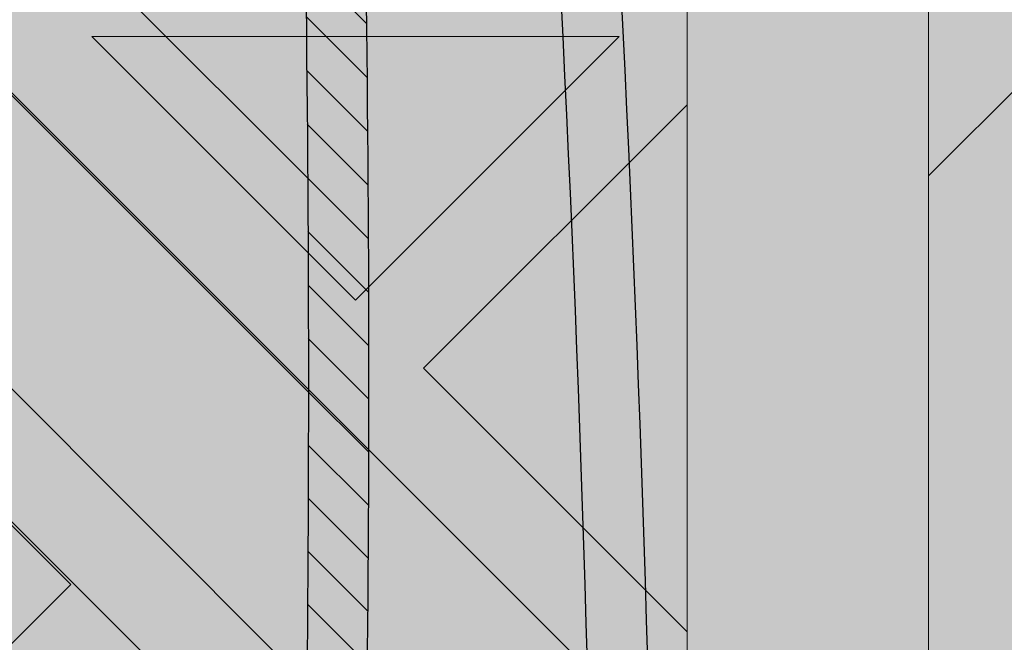
# Model space of a CAD drawing. Units: inches. Extents: x 844 to 2234, y 346 to 1084.
# Tile 36 of 93: x 1260.074 to 1262.676, y 697.583 to 699.229. Entities that reach past the tile are written whole.
import ezdxf

# ---------------------------------------------------------------- set-up
doc = ezdxf.new("R2010")
doc.units = ezdxf.units.IN
doc.header["$MEASUREMENT"] = 0
doc.layers.add('furniture', color=8, linetype='Continuous', lineweight=18)
doc.layers.add('RA-AP-01$0$INT', color=35, linetype='Continuous', lineweight=5)
doc.layers.add('RA-AP-01$0$FURN', color=3, linetype='Continuous')
doc.layers.add('RA-AP-01$0$WOOD', color=64, linetype='Continuous')

# ---------------------------------------------------------------- blocks, each defined once
blk = doc.blocks.new('A$C18D01794')
at = {"layer": 'RA-AP-01$0$INT'}
h = blk.add_hatch(color=256, dxfattribs=at)
h.paths.add_polyline_path([(4.50521, -7.5855), (4.46935, -7.54964), (4.50521, -7.51378), (4.50521, -7.38196), (4.46935, -7.34611), (4.50521, -7.31025), (4.50521, -7.17843), (4.46935, -7.14257), (4.50521, -7.10671), (4.47692, -7.10671), (4.45521, -7.12843), (4.43349, -7.10671), (4.40521, -7.10671), (4.44106, -7.14257), (4.40521, -7.17843), (4.40521, -7.31025), (4.44106, -7.34611), (4.40521, -7.38196), (4.40521, -7.51378), (4.44106, -7.54964), (4.40521, -7.5855), (4.40521, -7.71732), (4.44106, -7.75318), (4.40521, -7.78903), (4.40521, -8.00671), (4.64435, -8.00671), (4.68021, -7.97085), (4.71606, -8.00671), (4.86935, -8.00671), (4.90521, -7.97085), (4.94106, -8.00671), (5.09435, -8.00671), (5.13021, -7.97085), (5.16606, -8.00671), (5.40521, -8.00671), (5.40521, -7.78903), (5.36935, -7.75318), (5.40521, -7.71732), (5.40521, -7.5855), (5.36935, -7.54964), (5.40521, -7.51378), (5.40521, -7.38196), (5.36935, -7.34611), (5.40521, -7.31025), (5.40521, -7.17843), (5.36935, -7.14257), (5.40521, -7.10671), (5.37692, -7.10671), (5.35521, -7.12843), (5.33349, -7.10671), (5.30521, -7.10671), (5.34106, -7.14257), (5.30521, -7.17843), (5.30521, -7.31025), (5.34106, -7.34611), (5.30521, -7.38196), (5.30521, -7.51378), (5.34106, -7.54964), (5.30521, -7.5855), (5.30521, -7.71732), (5.34106, -7.75318), (5.30521, -7.78903), (5.30521, -7.90671), (5.16606, -7.90671), (5.13021, -7.94257), (5.09435, -7.90671), (4.94106, -7.90671), (4.90521, -7.94257), (4.86935, -7.90671), (4.71606, -7.90671), (4.68021, -7.94257), (4.64435, -7.90671), (4.50521, -7.90671), (4.50521, -7.78903), (4.46935, -7.75318), (4.50521, -7.71732)])
h.paths.add_polyline_path([(4.48521, -7.70903), (4.45521, -7.73903), (4.42521, -7.70903), (4.42521, -7.59378), (4.45521, -7.56378), (4.48521, -7.59378)], flags=16)
h.paths.add_polyline_path([(4.45521, -7.76732), (4.48521, -7.79732), (4.48521, -7.91257), (4.45521, -7.94257), (4.42521, -7.91257), (4.42521, -7.79732)], flags=16)
h.paths.add_polyline_path([(4.45521, -7.5355), (4.42521, -7.5055), (4.42521, -7.39025), (4.45521, -7.36025), (4.48521, -7.39025), (4.48521, -7.5055)], flags=16)
h.paths.add_polyline_path([(4.49935, -7.92671), (4.63606, -7.92671), (4.66606, -7.95671), (4.63606, -7.98671), (4.49935, -7.98671), (4.46935, -7.95671)], flags=16)
h.paths.add_polyline_path([(4.42521, -7.94085), (4.47106, -7.98671), (4.42521, -7.98671)], flags=16)
h.paths.add_polyline_path([(4.45521, -7.33196), (4.42521, -7.30196), (4.42521, -7.18671), (4.45521, -7.15671), (4.48521, -7.18671), (4.48521, -7.30196)], flags=16)
h.paths.add_polyline_path([(4.72435, -7.92671), (4.86106, -7.92671), (4.89106, -7.95671), (4.86106, -7.98671), (4.72435, -7.98671), (4.69435, -7.95671)], flags=16)
h.paths.add_polyline_path([(4.91935, -7.95671), (4.94935, -7.92671), (5.08606, -7.92671), (5.11606, -7.95671), (5.08606, -7.98671), (4.94935, -7.98671)], flags=16)
h.paths.add_polyline_path([(5.14435, -7.95671), (5.17435, -7.92671), (5.31106, -7.92671), (5.34106, -7.95671), (5.31106, -7.98671), (5.17435, -7.98671)], flags=16)
h.paths.add_polyline_path([(5.32521, -7.59378), (5.35521, -7.56378), (5.38521, -7.59378), (5.38521, -7.70903), (5.35521, -7.73903), (5.32521, -7.70903)], flags=16)
h.paths.add_polyline_path([(5.32521, -7.79732), (5.35521, -7.76732), (5.38521, -7.79732), (5.38521, -7.91257), (5.35521, -7.94257), (5.32521, -7.91257)], flags=16)
h.paths.add_polyline_path([(5.32521, -7.5055), (5.32521, -7.39025), (5.35521, -7.36025), (5.38521, -7.39025), (5.38521, -7.5055), (5.35521, -7.5355)], flags=16)
h.paths.add_polyline_path([(5.32521, -7.30196), (5.32521, -7.18671), (5.35521, -7.15671), (5.38521, -7.18671), (5.38521, -7.30196), (5.35521, -7.33196)], flags=16)
h.paths.add_polyline_path([(5.33935, -7.98671), (5.38521, -7.94085), (5.38521, -7.98671)], flags=16)
h = blk.add_hatch(color=256, dxfattribs=at)
h.paths.add_polyline_path([(4.46935, -7.14257), (4.50521, -7.17843), (4.50521, -7.10671)])
h.paths.add_polyline_path([(4.45521, -7.12843), (4.47692, -7.10671), (4.43349, -7.10671)])
h.paths.add_polyline_path([(4.40521, -7.17843), (4.44106, -7.14257), (4.40521, -7.10671)])
h.paths.add_polyline_path([(4.42521, -7.30196), (4.45521, -7.33196), (4.48521, -7.30196), (4.48521, -7.18671), (4.45521, -7.15671), (4.42521, -7.18671)])
h.paths.add_polyline_path([(4.50521, -7.38196), (4.50521, -7.31025), (4.46935, -7.34611)])
h.paths.add_polyline_path([(4.42521, -7.5055), (4.45521, -7.5355), (4.48521, -7.5055), (4.48521, -7.39025), (4.45521, -7.36025), (4.42521, -7.39025)])
h.paths.add_polyline_path([(4.42521, -7.70903), (4.45521, -7.73903), (4.48521, -7.70903), (4.48521, -7.59378), (4.45521, -7.56378), (4.42521, -7.59378)])
h.paths.add_polyline_path([(4.46935, -7.54964), (4.50521, -7.5855), (4.50521, -7.51378)])
h.paths.add_polyline_path([(4.40521, -7.5855), (4.44106, -7.54964), (4.40521, -7.51378)])
h.paths.add_polyline_path([(4.40521, -7.78903), (4.44106, -7.75318), (4.40521, -7.71732)])
h.paths.add_polyline_path([(4.46935, -7.75318), (4.50521, -7.78903), (4.50521, -7.71732)])
h.paths.add_polyline_path([(4.42521, -7.91257), (4.45521, -7.94257), (4.48521, -7.91257), (4.48521, -7.79732), (4.45521, -7.76732), (4.42521, -7.79732)])
h.paths.add_polyline_path([(4.42521, -7.98671), (4.47106, -7.98671), (4.42521, -7.94085)])
h.paths.add_polyline_path([(4.49935, -7.98671), (4.63606, -7.98671), (4.66606, -7.95671), (4.63606, -7.92671), (4.49935, -7.92671), (4.46935, -7.95671)])
h.paths.add_polyline_path([(4.68021, -7.94257), (4.71606, -7.90671), (4.64435, -7.90671)])
h.paths.add_polyline_path([(4.64435, -8.00671), (4.71606, -8.00671), (4.68021, -7.97085)])
h.paths.add_polyline_path([(4.72435, -7.98671), (4.86106, -7.98671), (4.89106, -7.95671), (4.86106, -7.92671), (4.72435, -7.92671), (4.69435, -7.95671)])
h.paths.add_polyline_path([(4.90521, -7.94257), (4.94106, -7.90671), (4.86935, -7.90671)])
h.paths.add_polyline_path([(4.86935, -8.00671), (4.94106, -8.00671), (4.90521, -7.97085)])
h.paths.add_polyline_path([(4.94935, -7.98671), (5.08606, -7.98671), (5.11606, -7.95671), (5.08606, -7.92671), (4.94935, -7.92671), (4.91935, -7.95671)])
h.paths.add_polyline_path([(5.13021, -7.94257), (5.16606, -7.90671), (5.09435, -7.90671)])
h.paths.add_polyline_path([(5.09435, -8.00671), (5.16606, -8.00671), (5.13021, -7.97085)])
h.paths.add_polyline_path([(5.17435, -7.98671), (5.31106, -7.98671), (5.34106, -7.95671), (5.31106, -7.92671), (5.17435, -7.92671), (5.14435, -7.95671)])
h.paths.add_polyline_path([(5.32521, -7.91257), (5.35521, -7.94257), (5.38521, -7.91257), (5.38521, -7.79732), (5.35521, -7.76732), (5.32521, -7.79732)])
h.paths.add_polyline_path([(5.33935, -7.98671), (5.38521, -7.98671), (5.38521, -7.94085)])
h.paths.add_polyline_path([(5.32521, -7.70903), (5.35521, -7.73903), (5.38521, -7.70903), (5.38521, -7.59378), (5.35521, -7.56378), (5.32521, -7.59378)])
h.paths.add_polyline_path([(5.30521, -7.78903), (5.34106, -7.75318), (5.30521, -7.71732)])
h.paths.add_polyline_path([(5.36935, -7.75318), (5.40521, -7.78903), (5.40521, -7.71732)])
h.paths.add_polyline_path([(5.40521, -7.5855), (5.40521, -7.51378), (5.36935, -7.54964)])
h.paths.add_polyline_path([(5.30521, -7.5855), (5.34106, -7.54964), (5.30521, -7.51378)])
h.paths.add_polyline_path([(5.32521, -7.5055), (5.35521, -7.5355), (5.38521, -7.5055), (5.38521, -7.39025), (5.35521, -7.36025), (5.32521, -7.39025)])
h.paths.add_polyline_path([(5.30521, -7.38196), (5.34106, -7.34611), (5.30521, -7.31025)])
h.paths.add_polyline_path([(5.32521, -7.30196), (5.35521, -7.33196), (5.38521, -7.30196), (5.38521, -7.18671), (5.35521, -7.15671), (5.32521, -7.18671)])
h.paths.add_polyline_path([(5.40458, -7.38134, -0.001218), (5.40521, -7.38111), (5.40521, -7.31025), (5.36935, -7.34611)])
h.paths.add_polyline_path([(5.36935, -7.14257), (5.40521, -7.17843), (5.40521, -7.10671)])
h.paths.add_polyline_path([(5.35521, -7.12843), (5.37692, -7.10671), (5.33349, -7.10671)])
h.paths.add_polyline_path([(5.30521, -7.17843), (5.34106, -7.14257), (5.30521, -7.10671)])
blk.add_hatch(color=256, dxfattribs=at).paths.add_polyline_path([(4.50521, -7.90671), (5.30521, -7.90671), (5.30521, -7.10671), (5.25521, -7.10671), (5.25521, -7.85671), (4.55521, -7.85671), (4.55521, -7.10671), (4.50521, -7.10671)])
h = blk.add_hatch(color=256, dxfattribs=at)
h.paths.add_polyline_path([(4.58592, -7.85671), (4.6142, -7.85671), (4.66885, -7.80207), (4.72349, -7.85671), (4.77177, -7.85671), (4.82642, -7.80207), (4.86278, -7.83843), (4.8445, -7.85671), (4.86278, -7.85671), (4.90521, -7.81429), (4.94763, -7.85671), (4.96592, -7.85671), (4.94763, -7.83843), (4.98399, -7.80207), (5.03864, -7.85671), (5.08692, -7.85671), (5.14157, -7.80207), (5.19621, -7.85671), (5.2245, -7.85671), (4.90521, -7.53742)])
h.paths.add_polyline_path([(4.89521, -7.57571), (4.89521, -7.685), (4.84056, -7.63035)], flags=16)
h.paths.add_polyline_path([(4.91521, -7.57571), (4.96985, -7.63035), (4.91521, -7.685)], flags=16)
h.paths.add_polyline_path([(4.82642, -7.64449), (4.88106, -7.69914), (4.77177, -7.69914)], flags=16)
h.paths.add_polyline_path([(4.98399, -7.64449), (5.03864, -7.69914), (4.92935, -7.69914)], flags=16)
h.paths.add_polyline_path([(4.88106, -7.71914), (4.82642, -7.77378), (4.77177, -7.71914)], flags=16)
h.paths.add_polyline_path([(4.92935, -7.71914), (5.03864, -7.71914), (4.98399, -7.77378)], flags=16)
h.paths.add_polyline_path([(4.89521, -7.73328), (4.89521, -7.806), (4.87692, -7.82429), (4.84056, -7.78793)], flags=16)
h.paths.add_polyline_path([(4.91521, -7.73328), (4.96985, -7.78793), (4.93349, -7.82429), (4.91521, -7.806)], flags=16)
h.paths.add_polyline_path([(4.75763, -7.73328), (4.81228, -7.78793), (4.75763, -7.84257)], flags=16)
h.paths.add_polyline_path([(4.73763, -7.73328), (4.73763, -7.84257), (4.68299, -7.78793)], flags=16)
h.paths.add_polyline_path([(5.05278, -7.73328), (5.05278, -7.84257), (4.99814, -7.78793)], flags=16)
h.paths.add_polyline_path([(5.07278, -7.73328), (5.12742, -7.78793), (5.07278, -7.84257)], flags=16)
h.paths.add_polyline_path([(4.93592, -7.50671), (5.25521, -7.826), (5.25521, -7.79772), (5.20056, -7.74307), (5.25521, -7.68843), (5.25521, -7.64014), (5.20056, -7.5855), (5.23692, -7.54914), (5.25521, -7.56742), (5.25521, -7.54914), (5.21278, -7.50671), (5.25521, -7.46429), (5.25521, -7.446), (5.23692, -7.46429), (5.20056, -7.42793), (5.25521, -7.37328), (5.25521, -7.325), (5.20056, -7.27035), (5.25521, -7.21571), (5.25521, -7.18742)])
h.paths.add_polyline_path([(5.04299, -7.42793), (5.09763, -7.37328), (5.09763, -7.48257)], flags=16)
h.paths.add_polyline_path([(5.02885, -7.44207), (5.08349, -7.49671), (4.9742, -7.49671)], flags=16)
h.paths.add_polyline_path([(5.11763, -7.37328), (5.17228, -7.42793), (5.11763, -7.48257)], flags=16)
h.paths.add_polyline_path([(5.08349, -7.51671), (5.02885, -7.57136), (4.9742, -7.51671)], flags=16)
h.paths.add_polyline_path([(5.13177, -7.35914), (5.18642, -7.41378), (5.24106, -7.35914)], flags=17)
h.paths.add_polyline_path([(5.13177, -7.49671), (5.18642, -7.44207), (5.22278, -7.47843), (5.2045, -7.49671)], flags=16)
h.paths.add_polyline_path([(5.09763, -7.53085), (5.09763, -7.64014), (5.04299, -7.5855)], flags=16)
h.paths.add_polyline_path([(5.13177, -7.33914), (5.24106, -7.33914), (5.18642, -7.28449)], flags=17)
h.paths.add_polyline_path([(5.13177, -7.51671), (5.2045, -7.51671), (5.22278, -7.535), (5.18642, -7.57136)], flags=16)
h.paths.add_polyline_path([(5.11763, -7.53085), (5.17228, -7.5855), (5.11763, -7.64014)], flags=16)
h.paths.add_polyline_path([(5.18642, -7.59964), (5.24106, -7.65429), (5.13177, -7.65429)], flags=16)
h.paths.add_polyline_path([(5.13177, -7.67429), (5.24106, -7.67429), (5.18642, -7.72893)], flags=16)
h.paths.add_polyline_path([(5.25521, -7.126), (5.25521, -7.10671), (4.55521, -7.10671), (4.55521, -7.126), (4.90521, -7.476)])
h.paths.add_polyline_path([(4.98399, -7.36893), (4.92935, -7.31429), (5.03864, -7.31429)], flags=16)
h.paths.add_polyline_path([(4.96985, -7.38307), (4.91521, -7.43772), (4.91521, -7.32843)], flags=16)
h.paths.add_polyline_path([(4.92935, -7.29429), (4.98399, -7.23964), (5.03864, -7.29429)], flags=16)
h.paths.add_polyline_path([(5.05278, -7.28014), (4.99814, -7.2255), (5.05278, -7.17085)], flags=16)
h.paths.add_polyline_path([(5.07278, -7.28014), (5.07278, -7.17085), (5.12742, -7.2255)], flags=16)
h.paths.add_polyline_path([(4.89521, -7.43772), (4.84056, -7.38307), (4.89521, -7.32843)], flags=16)
h.paths.add_polyline_path([(4.91521, -7.28014), (4.91521, -7.20742), (4.93349, -7.18914), (4.96985, -7.2255)], flags=16)
h.paths.add_polyline_path([(4.88106, -7.31429), (4.82642, -7.36893), (4.77177, -7.31429)], flags=16)
h.paths.add_polyline_path([(4.89521, -7.28014), (4.84056, -7.2255), (4.87692, -7.18914), (4.89521, -7.20742)], flags=16)
h.paths.add_polyline_path([(4.98399, -7.21136), (4.94763, -7.175), (4.96592, -7.15671), (5.03864, -7.15671)], flags=16)
h.paths.add_polyline_path([(4.88106, -7.29429), (4.77177, -7.29429), (4.82642, -7.23964)], flags=16)
h.paths.add_polyline_path([(4.90521, -7.19914), (4.86278, -7.15671), (4.94763, -7.15671)], flags=16)
h.paths.add_polyline_path([(5.14157, -7.21136), (5.08692, -7.15671), (5.19621, -7.15671)], flags=16)
h.paths.add_polyline_path([(4.82642, -7.21136), (4.77177, -7.15671), (4.8445, -7.15671), (4.86278, -7.175)], flags=16)
h.paths.add_polyline_path([(4.81228, -7.2255), (4.75763, -7.28014), (4.75763, -7.17085)], flags=16)
h.paths.add_polyline_path([(4.73763, -7.28014), (4.68299, -7.2255), (4.73763, -7.17085)], flags=16)
h.paths.add_polyline_path([(4.72349, -7.15671), (4.66885, -7.21136), (4.6142, -7.15671)], flags=16)
h.paths.add_polyline_path([(4.59763, -7.50671), (4.55521, -7.54914), (4.55521, -7.56742), (4.57349, -7.54914), (4.60985, -7.5855), (4.55521, -7.64014), (4.55521, -7.68843), (4.60985, -7.74307), (4.55521, -7.79772), (4.55521, -7.826), (4.8745, -7.50671), (4.55521, -7.18742), (4.55521, -7.21571), (4.60985, -7.27035), (4.55521, -7.325), (4.55521, -7.37328), (4.60985, -7.42793), (4.57349, -7.46429), (4.55521, -7.446), (4.55521, -7.46429)])
h.paths.add_polyline_path([(4.71278, -7.48257), (4.71278, -7.37328), (4.76742, -7.42793)], flags=16)
h.paths.add_polyline_path([(4.72692, -7.49671), (4.78157, -7.44207), (4.83621, -7.49671)], flags=16)
h.paths.add_polyline_path([(4.69278, -7.48257), (4.63814, -7.42793), (4.69278, -7.37328)], flags=16)
h.paths.add_polyline_path([(4.72692, -7.51671), (4.83621, -7.51671), (4.78157, -7.57136)], flags=16)
h.paths.add_polyline_path([(4.67864, -7.49671), (4.60592, -7.49671), (4.58763, -7.47843), (4.62399, -7.44207)], flags=16)
h.paths.add_polyline_path([(4.71278, -7.53085), (4.76742, -7.5855), (4.71278, -7.64014)], flags=16)
h.paths.add_polyline_path([(4.67864, -7.51671), (4.62399, -7.57136), (4.58763, -7.535), (4.60592, -7.51671)], flags=16)
h.paths.add_polyline_path([(4.69278, -7.53085), (4.69278, -7.64014), (4.63814, -7.5855)], flags=16)
h.paths.add_polyline_path([(4.62399, -7.41378), (4.67864, -7.35914), (4.56935, -7.35914)], flags=17)
h.paths.add_polyline_path([(4.62399, -7.59964), (4.67864, -7.65429), (4.56935, -7.65429)], flags=16)
h.paths.add_polyline_path([(4.67864, -7.33914), (4.62399, -7.28449), (4.56935, -7.33914)], flags=17)
h.paths.add_polyline_path([(4.67864, -7.67429), (4.62399, -7.72893), (4.56935, -7.67429)], flags=16)
h = blk.add_hatch(color=256, dxfattribs=at)
h.paths.add_polyline_path([(4.90521, -7.53742), (4.8745, -7.50671), (4.55521, -7.826), (4.55521, -7.85671), (4.58592, -7.85671)])
h.paths.add_polyline_path([(4.93592, -7.50671), (4.90521, -7.53742), (5.2245, -7.85671), (5.25521, -7.85671), (5.25521, -7.826)])
h.paths.add_polyline_path([(5.25521, -7.18742), (5.25521, -7.126), (4.90521, -7.476), (4.93592, -7.50671)])
h.paths.add_polyline_path([(4.8745, -7.50671), (4.90521, -7.476), (4.55521, -7.126), (4.55521, -7.18742)])
h = blk.add_hatch(color=256, dxfattribs=at)
h.paths.add_polyline_path([(4.89521, -7.32843), (4.84056, -7.38307), (4.89521, -7.43772)])
h.paths.add_polyline_path([(4.91521, -7.43772), (4.96985, -7.38307), (4.91521, -7.32843)])
h.paths.add_polyline_path([(4.92935, -7.31429), (4.98399, -7.36893), (5.03864, -7.31429)])
h.paths.add_polyline_path([(5.03864, -7.29429), (4.98399, -7.23964), (4.92935, -7.29429)])
h.paths.add_polyline_path([(4.96985, -7.2255), (4.93349, -7.18914), (4.91521, -7.20742), (4.91521, -7.28014)])
h.paths.add_polyline_path([(4.96592, -7.15671), (4.94763, -7.175), (4.98399, -7.21136), (5.03864, -7.15671)])
h.paths.add_polyline_path([(4.99814, -7.2255), (5.05278, -7.28014), (5.05278, -7.17085)])
h.paths.add_polyline_path([(5.07278, -7.28014), (5.12742, -7.2255), (5.07278, -7.17085)])
h.paths.add_polyline_path([(5.19621, -7.15671), (5.08692, -7.15671), (5.14157, -7.21136)])
h.paths.add_polyline_path([(4.86278, -7.15671), (4.90521, -7.19914), (4.94763, -7.15671)])
h.paths.add_polyline_path([(4.89521, -7.28014), (4.89521, -7.20742), (4.87692, -7.18914), (4.84056, -7.2255)])
h.paths.add_polyline_path([(4.82642, -7.23964), (4.77177, -7.29429), (4.88106, -7.29429)])
h.paths.add_polyline_path([(4.77177, -7.31429), (4.82642, -7.36893), (4.88106, -7.31429)])
h.paths.add_polyline_path([(4.75763, -7.28014), (4.81228, -7.2255), (4.75763, -7.17085)])
h.paths.add_polyline_path([(4.86278, -7.175), (4.8445, -7.15671), (4.77177, -7.15671), (4.82642, -7.21136)])
h.paths.add_polyline_path([(4.68299, -7.2255), (4.73763, -7.28014), (4.73763, -7.17085)])
h.paths.add_polyline_path([(4.72349, -7.15671), (4.6142, -7.15671), (4.66885, -7.21136)])
h = blk.add_hatch(color=256, dxfattribs=at)
h.paths.add_polyline_path([(4.78157, -7.44207), (4.83621, -7.49671), (4.72692, -7.49671)])
h.paths.add_polyline_path([(4.83621, -7.51671), (4.78157, -7.57136), (4.72692, -7.51671)])
h.paths.add_polyline_path([(4.76742, -7.5855), (4.71278, -7.64014), (4.71278, -7.53085)])
h.paths.add_polyline_path([(4.69278, -7.53085), (4.69278, -7.64014), (4.63814, -7.5855)])
h.paths.add_polyline_path([(4.67864, -7.51671), (4.62399, -7.57136), (4.58763, -7.535), (4.60592, -7.51671)])
h.paths.add_polyline_path([(4.57349, -7.54914), (4.60985, -7.5855), (4.55521, -7.64014), (4.55521, -7.56742)])
h.paths.add_polyline_path([(4.62399, -7.59964), (4.67864, -7.65429), (4.56935, -7.65429)])
h.paths.add_polyline_path([(4.67864, -7.67429), (4.62399, -7.72893), (4.56935, -7.67429)])
h.paths.add_polyline_path([(4.60985, -7.74307), (4.55521, -7.79772), (4.55521, -7.68843)])
h.paths.add_polyline_path([(4.59763, -7.50671), (4.55521, -7.54914), (4.55521, -7.46429)])
h.paths.add_polyline_path([(4.67864, -7.49671), (4.60592, -7.49671), (4.58763, -7.47843), (4.62399, -7.44207)])
h.paths.add_polyline_path([(4.69278, -7.37328), (4.69278, -7.48257), (4.63814, -7.42793)])
h.paths.add_polyline_path([(4.76742, -7.42793), (4.71278, -7.48257), (4.71278, -7.37328)])
h.paths.add_polyline_path([(4.67864, -7.35914), (4.62399, -7.41378), (4.56935, -7.35914)])
h.paths.add_polyline_path([(4.60985, -7.42793), (4.57349, -7.46429), (4.55521, -7.446), (4.55521, -7.37328)])
h.paths.add_polyline_path([(4.62399, -7.28449), (4.67864, -7.33914), (4.56935, -7.33914)])
h.paths.add_polyline_path([(4.60985, -7.27035), (4.55521, -7.325), (4.55521, -7.21571)])
for p, q in [((4.55521, -7.10671), (4.55521, -7.85671)), ((4.90521, -7.476), (4.55521, -7.126)), ((4.73763, -7.17085), (4.68299, -7.2255)), ((4.8745, -7.50671), (4.55521, -7.18742)), ((4.55521, -7.21571), (4.60985, -7.27035)), ((4.55521, -7.325), (4.55521, -7.21571)), ((4.68299, -7.2255), (4.73763, -7.28014)), ((4.55521, -7.325), (4.60985, -7.27035)), ((4.56935, -7.33914), (4.62399, -7.28449)), ((4.62399, -7.28449), (4.67864, -7.33914)), ((4.50521, -7.31025), (4.46935, -7.34611)), ((4.67864, -7.33914), (4.56935, -7.33914))]:
    blk.add_line(p, q, dxfattribs=at)
blk.add_lwpolyline([(5.30521, -7.10671), (5.30521, -7.90671), (4.50521, -7.90671), (4.50521, -7.10671)], dxfattribs=at)
blk = doc.blocks.new('A$C32926AE1')
at = {"layer": 'RA-AP-01$0$WOOD'}
h = blk.add_hatch(color=256, dxfattribs=at)
h.dxf.hatch_style = 1
h.paths.add_polyline_path([(5.15743, 4.57348, -0.100949), (5.1554, 4.59337, -0.184266), (5.17225, 4.6388, 0.205661), (5.17956, 4.66132, 0.361434), (5.13435, 4.70652, 0.205661), (5.11183, 4.69921, -0.184266), (5.0664, 4.68237, -0.105531), (5.04566, 4.68467, 0.156764), (4.76389, 4.68467, -0.105531), (4.74314, 4.68237, -0.184266), (4.69771, 4.69921, 0.205661), (4.67519, 4.70652, 0.361434), (4.62998, 4.66132, 0.205661), (4.63729, 4.6388, -0.184266), (4.65414, 4.59337, -0.100949), (4.65211, 4.57348, 0.02141), (4.62975, 4.15671, 0.02141), (4.65211, 3.73994, -0.100949), (4.65414, 3.72006, -0.184266), (4.63729, 3.67463, 0.205661), (4.62998, 3.65211, 0.361434), (4.67519, 3.6069, 0.205661), (4.69771, 3.61421, -0.184266), (4.74314, 3.63106, -0.105531), (4.76389, 3.62875, 0.156764), (5.04566, 3.62875, -0.105531), (5.0664, 3.63106, -0.184266), (5.11183, 3.61421, 0.205661), (5.13435, 3.6069, 0.361434), (5.17956, 3.65211, 0.205661), (5.17225, 3.67463, -0.184266), (5.1554, 3.72006, -0.100949), (5.15743, 3.73994, 0.02141), (5.17979, 4.15671, 0.02141)])
h.paths.add_polyline_path([(4.63975, 4.15671, 0.021354), (4.66197, 3.74189, -0.094076), (4.66414, 3.71961, -0.182482), (4.64481, 3.66804, 0.205661), (4.63994, 3.65302, 0.361434), (4.67611, 3.61686, 0.205661), (4.69112, 3.62173, -0.182482), (4.7427, 3.64106, -0.102989), (4.76699, 3.63826, 0.156709), (5.04255, 3.63826, -0.102989), (5.06685, 3.64106, -0.182482), (5.11842, 3.62173, 0.205661), (5.13344, 3.61686, 0.361434), (5.1696, 3.65302, 0.205661), (5.16473, 3.66804, -0.182482), (5.1454, 3.71961, -0.094076), (5.14757, 3.74189, 0.021354), (5.16979, 4.15671, 0.021354), (5.14757, 4.57154, -0.094076), (5.1454, 4.59381, -0.182482), (5.16473, 4.64539, 0.205661), (5.1696, 4.6604, 0.361434), (5.13344, 4.69657, 0.205661), (5.11842, 4.69169, -0.182482), (5.06685, 4.67236, -0.102989), (5.04255, 4.67517, 0.156709), (4.76699, 4.67517, -0.102989), (4.7427, 4.67236, -0.182482), (4.69112, 4.69169, 0.205661), (4.67611, 4.69657, 0.361434), (4.63994, 4.6604, 0.205661), (4.64481, 4.64539, -0.182482), (4.66414, 4.59381, -0.094076), (4.66197, 4.57154, 0.021354)], flags=16)
h.paths.add_polyline_path([(5.12979, 4.43217, -0.014166), (5.13015, 4.15693, -0.014166), (5.12979, 3.88169, -0.078525), (5.1098, 3.75514, 0.094597), (5.10541, 3.7179, 0.104317), (5.11607, 3.67039, 0.104317), (5.06856, 3.68105, 0.094597), (5.03132, 3.67666, -0.158024), (4.77823, 3.67666, 0.094597), (4.74098, 3.68105, 0.104317), (4.69347, 3.67039, 0.104317), (4.70413, 3.7179, 0.094597), (4.69975, 3.75514, -0.078525), (4.67975, 3.88169, -0.014166), (4.67939, 4.15693, -0.014166), (4.67975, 4.43217, -0.078525), (4.69975, 4.55871, 0.094597), (4.70413, 4.59596, 0.104317), (4.69347, 4.64347, 0.104317), (4.74098, 4.6328, 0.094597), (4.77823, 4.63719, -0.158024), (5.03132, 4.63719, 0.094597), (5.06856, 4.6328, 0.104317), (5.11607, 4.64347, 0.104317), (5.10541, 4.59596, 0.094597), (5.1098, 4.55871, -0.078525)], flags=0)
h.paths.add_polyline_path([(5.11979, 4.43226, -0.0142), (5.12016, 4.15693, -0.0142), (5.11979, 3.8816, -0.078489), (5.10027, 3.75819, 0.094014), (5.09541, 3.71748, 0.060627), (5.09962, 3.68684, 0.060627), (5.06898, 3.69105, 0.094014), (5.02827, 3.68619, -0.158071), (4.78127, 3.68619, 0.094014), (4.74056, 3.69105, 0.060627), (4.70993, 3.68684, 0.060627), (4.71413, 3.71748, 0.094014), (4.70927, 3.75819, -0.078489), (4.68975, 3.8816, -0.0142), (4.68939, 4.15693, -0.0142), (4.68975, 4.43226, -0.078489), (4.70927, 4.55566, 0.094014), (4.71413, 4.59638, 0.060627), (4.70993, 4.62701, 0.060627), (4.74056, 4.62281, 0.094014), (4.78127, 4.62767, -0.158071), (5.02827, 4.62767, 0.094014), (5.06898, 4.62281, 0.060627), (5.09962, 4.62701, 0.060627), (5.09541, 4.59638, 0.094014), (5.10027, 4.55566, -0.078489)], flags=0)
h.paths.add_polyline_path([(5.06979, 4.43022, -0.014242), (5.07017, 4.15693, -0.014242), (5.06979, 3.88364, -0.080061), (5.05266, 3.77346, 0.052642), (5.04591, 3.74055, 0.052642), (5.013, 3.7338, -0.158303), (4.79655, 3.7338, 0.052642), (4.76363, 3.74055, 0.052642), (4.75688, 3.77346, -0.080061), (4.73975, 3.88364, -0.014242), (4.73937, 4.15693, -0.014242), (4.73975, 4.43022, -0.080061), (4.75688, 4.54039, 0.052642), (4.76363, 4.5733, 0.052642), (4.79655, 4.58006, -0.158303), (5.013, 4.58006, 0.052642), (5.04591, 4.5733, 0.052642), (5.05266, 4.54039, -0.080061)], flags=0)
h.paths.add_polyline_path([(5.04979, 4.43038, -0.01431), (5.05018, 4.15693, -0.01431), (5.04979, 3.88347, -0.080069), (5.03362, 3.77958, 0.030626), (5.02824, 3.75822, 0.030626), (5.00688, 3.75284, -0.158398), (4.80266, 3.75284, 0.030626), (4.7813, 3.75822, 0.030626), (4.77592, 3.77958, -0.080069), (4.75975, 3.88347, -0.01431), (4.75936, 4.15693, -0.01431), (4.75975, 4.43038, -0.080069), (4.77592, 4.53427, 0.030626), (4.7813, 4.55564, 0.030626), (4.80266, 4.56102, -0.158398), (5.00688, 4.56102, 0.030626), (5.02824, 4.55564, 0.030626), (5.03362, 4.53427, -0.080069)], flags=0)
h.paths.add_polyline_path([(4.99977, 4.42817, -0.014344), (5.0002, 4.15693, -0.014344), (4.99977, 3.88568, -0.078464), (4.98736, 3.7991, -0.150605), (4.82219, 3.7991, -0.078464), (4.80978, 3.88568, -0.014344), (4.80934, 4.15693, -0.014344), (4.80978, 4.42817, -0.078464), (4.82219, 4.51475, -0.150605), (4.98736, 4.51475, -0.078464)], flags=0)
h.paths.add_polyline_path([(4.97976, 4.42764, -0.014377), (4.98021, 4.15693, -0.014377), (4.97976, 3.88621, -0.068924), (4.97118, 3.81528, -0.129665), (4.83836, 3.81528, -0.068924), (4.82979, 3.88621, -0.014377), (4.82934, 4.15693, -0.014377), (4.82979, 4.42764, -0.068924), (4.83836, 4.49858, -0.129665), (4.97118, 4.49858, -0.068924)], flags=0)
h = blk.add_hatch(color=256, dxfattribs=at)
h.dxf.hatch_style = 1
h.paths.add_polyline_path([(5.1454, 4.59381, -0.182482), (5.16473, 4.64539, 0.205661), (5.1696, 4.6604, 0.361434), (5.13344, 4.69657, 0.205661), (5.11842, 4.69169, -0.182482), (5.06685, 4.67236, -0.102989), (5.04255, 4.67517, 0.156709), (4.76699, 4.67517, -0.102989), (4.7427, 4.67236, -0.182482), (4.69112, 4.69169, 0.205661), (4.67611, 4.69657, 0.361434), (4.63994, 4.6604, 0.205661), (4.64481, 4.64539, -0.182482), (4.66414, 4.59381, -0.094076), (4.66197, 4.57154, 0.021354), (4.63975, 4.15671, 0.021354), (4.66197, 3.74189, -0.094076), (4.66414, 3.71961, -0.182482), (4.64481, 3.66804, 0.205661), (4.63994, 3.65302, 0.361434), (4.67611, 3.61686, 0.205661), (4.69112, 3.62173, -0.182482), (4.7427, 3.64106, -0.102989), (4.76699, 3.63826, 0.156709), (5.04255, 3.63826, -0.102989), (5.06685, 3.64106, -0.182482), (5.11842, 3.62173, 0.205661), (5.13344, 3.61686, 0.361434), (5.1696, 3.65302, 0.205661), (5.16473, 3.66804, -0.182482), (5.1454, 3.71961, -0.094076), (5.14757, 3.74189, 0.021354), (5.16979, 4.15671, 0.021354), (5.14757, 4.57154, -0.094076)])
h.paths.add_polyline_path([(5.1098, 4.55871, -0.078525), (5.12979, 4.43217, -0.014166), (5.13015, 4.15693, -0.014166), (5.12979, 3.88169, -0.078525), (5.1098, 3.75514, 0.094597), (5.10541, 3.7179, 0.104317), (5.11607, 3.67039, 0.104317), (5.06856, 3.68105, 0.094597), (5.03132, 3.67666, -0.158024), (4.77823, 3.67666, 0.094597), (4.74098, 3.68105, 0.104317), (4.69347, 3.67039, 0.104317), (4.70413, 3.7179, 0.094597), (4.69975, 3.75514, -0.078525), (4.67975, 3.88169, -0.014166), (4.67939, 4.15693, -0.014166), (4.67975, 4.43217, -0.078525), (4.69975, 4.55871, 0.094597), (4.70413, 4.59596, 0.104317), (4.69347, 4.64347, 0.104317), (4.74098, 4.6328, 0.094597), (4.77823, 4.63719, -0.158024), (5.03132, 4.63719, 0.094597), (5.06856, 4.6328, 0.104317), (5.11607, 4.64347, 0.104317), (5.10541, 4.59596, 0.094597)], flags=16)
h.paths.add_polyline_path([(5.10027, 4.55566, -0.078489), (5.11979, 4.43226, -0.0142), (5.12016, 4.15693, -0.0142), (5.11979, 3.8816, -0.078489), (5.10027, 3.75819, 0.094014), (5.09541, 3.71748, 0.060627), (5.09962, 3.68684, 0.060627), (5.06898, 3.69105, 0.094014), (5.02827, 3.68619, -0.158071), (4.78127, 3.68619, 0.094014), (4.74056, 3.69105, 0.060627), (4.70993, 3.68684, 0.060627), (4.71413, 3.71748, 0.094014), (4.70927, 3.75819, -0.078489), (4.68975, 3.8816, -0.0142), (4.68939, 4.15693, -0.0142), (4.68975, 4.43226, -0.078489), (4.70927, 4.55566, 0.094014), (4.71413, 4.59638, 0.060627), (4.70993, 4.62701, 0.060627), (4.74056, 4.62281, 0.094014), (4.78127, 4.62767, -0.158071), (5.02827, 4.62767, 0.094014), (5.06898, 4.62281, 0.060627), (5.09962, 4.62701, 0.060627), (5.09541, 4.59638, 0.094014)], flags=0)
h.paths.add_polyline_path([(5.04591, 4.5733, 0.052642), (5.05266, 4.54039, -0.080061), (5.06979, 4.43022, -0.014242), (5.07017, 4.15693, -0.014242), (5.06979, 3.88364, -0.080061), (5.05266, 3.77346, 0.052642), (5.04591, 3.74055, 0.052642), (5.013, 3.7338, -0.158303), (4.79655, 3.7338, 0.052642), (4.76363, 3.74055, 0.052642), (4.75688, 3.77346, -0.080061), (4.73975, 3.88364, -0.014242), (4.73937, 4.15693, -0.014242), (4.73975, 4.43022, -0.080061), (4.75688, 4.54039, 0.052642), (4.76363, 4.5733, 0.052642), (4.79655, 4.58006, -0.158303), (5.013, 4.58006, 0.052642)], flags=0)
h.paths.add_polyline_path([(5.02824, 4.55564, 0.030626), (5.03362, 4.53427, -0.080069), (5.04979, 4.43038, -0.01431), (5.05018, 4.15693, -0.01431), (5.04979, 3.88347, -0.080069), (5.03362, 3.77958, 0.030626), (5.02824, 3.75822, 0.030626), (5.00688, 3.75284, -0.158398), (4.80266, 3.75284, 0.030626), (4.7813, 3.75822, 0.030626), (4.77592, 3.77958, -0.080069), (4.75975, 3.88347, -0.01431), (4.75936, 4.15693, -0.01431), (4.75975, 4.43038, -0.080069), (4.77592, 4.53427, 0.030626), (4.7813, 4.55564, 0.030626), (4.80266, 4.56102, -0.158398), (5.00688, 4.56102, 0.030626)], flags=0)
h.paths.add_polyline_path([(4.98736, 4.51475, -0.078464), (4.99977, 4.42817, -0.014344), (5.0002, 4.15693, -0.014344), (4.99977, 3.88568, -0.078464), (4.98736, 3.7991, -0.150605), (4.82219, 3.7991, -0.078464), (4.80978, 3.88568, -0.014344), (4.80934, 4.15693, -0.014344), (4.80978, 4.42817, -0.078464), (4.82219, 4.51475, -0.150605)], flags=0)
h.paths.add_polyline_path([(4.97118, 4.49858, -0.068924), (4.97976, 4.42764, -0.014377), (4.98021, 4.15693, -0.014377), (4.97976, 3.88621, -0.068924), (4.97118, 3.81528, -0.129665), (4.83836, 3.81528, -0.068924), (4.82979, 3.88621, -0.014377), (4.82934, 4.15693, -0.014377), (4.82979, 4.42764, -0.068924), (4.83836, 4.49858, -0.129665)], flags=0)
h = blk.add_hatch(dxfattribs=at)
h.set_pattern_fill('ANSI31', color=256, scale=0.05, style=0)
h.paths.add_polyline_path([(5.13015, 4.15693, 0.014166), (5.12979, 4.43217, 0.077783), (5.11017, 4.55756, -0.097652), (5.10541, 4.59596, -0.104317), (5.11607, 4.64347), (5.09962, 4.62701, 0.060627), (5.09541, 4.59638, 0.094014), (5.10027, 4.55566, -0.078489), (5.11979, 4.43226, -0.0142), (5.12016, 4.15693, -0.0142), (5.11979, 3.8816, -0.078489), (5.10027, 3.75819, 0.094014), (5.09541, 3.71748, 0.060627), (5.09962, 3.68684), (5.11607, 3.67039, -0.104317), (5.10541, 3.7179, -0.097652), (5.11017, 3.7563, 0.077783), (5.12979, 3.88169, 0.014166)])
h.paths.add_polyline_path([(5.03016, 3.67629, -0.097652), (5.06856, 3.68105, -0.104317), (5.11607, 3.67039), (5.09962, 3.68684, 0.060627), (5.06898, 3.69105, 0.094014), (5.02827, 3.68619, -0.158071), (4.78127, 3.68619, 0.094014), (4.74056, 3.69105, 0.060627), (4.70993, 3.68684), (4.69347, 3.67039, -0.104317), (4.74098, 3.68105, -0.097652), (4.77938, 3.67629, 0.156513)])
h.paths.add_polyline_path([(4.68975, 3.8816, -0.0142), (4.68939, 4.15693, -0.0142), (4.68975, 4.43226, -0.078489), (4.70927, 4.55566, 0.094014), (4.71413, 4.59638, 0.060627), (4.70993, 4.62701), (4.69347, 4.64347, -0.104317), (4.70413, 4.59596, -0.097652), (4.69937, 4.55756, 0.077783), (4.67975, 4.43217, 0.014166), (4.67939, 4.15693, 0.014166), (4.67975, 3.88169, 0.077783), (4.69937, 3.7563, -0.097652), (4.70413, 3.7179, -0.104317), (4.69347, 3.67039), (4.70993, 3.68684, 0.060627), (4.71413, 3.71748, 0.094014), (4.70927, 3.75819, -0.078489)])
h.paths.add_polyline_path([(4.77938, 4.63756, -0.097652), (4.74098, 4.6328, -0.104317), (4.69347, 4.64347), (4.70993, 4.62701, 0.060627), (4.74056, 4.62281, 0.094014), (4.78127, 4.62767, -0.158071), (5.02827, 4.62767, 0.094014), (5.06898, 4.62281, 0.060627), (5.09962, 4.62701), (5.11607, 4.64347, -0.104317), (5.06856, 4.6328, -0.097652), (5.03016, 4.63756, 0.156513)])
h = blk.add_hatch(dxfattribs=at)
h.set_pattern_fill('ANSI32', color=256, scale=0.2, style=0)
h.paths.add_polyline_path([(5.11979, 4.43226, 0.077702), (5.10066, 4.55447, -0.09689), (5.09541, 4.59638, -0.060627), (5.09962, 4.62701, -0.060627), (5.06898, 4.62281, -0.09689), (5.02707, 4.62805, 0.156466), (4.78247, 4.62805, -0.09689), (4.74056, 4.62281, -0.060627), (4.70993, 4.62701, -0.060627), (4.71413, 4.59638, -0.09689), (4.70888, 4.55447, 0.077702), (4.68975, 4.43226, 0.0142), (4.68939, 4.15693, 0.0142), (4.68975, 3.8816, 0.077702), (4.70888, 3.75939, -0.09689), (4.71413, 3.71748, -0.060627), (4.70993, 3.68684, -0.060627), (4.74056, 3.69105, -0.09689), (4.78247, 3.6858, 0.156466), (5.02707, 3.6858, -0.09689), (5.06898, 3.69105, -0.060627), (5.09962, 3.68684, -0.060627), (5.09541, 3.71748, -0.09689), (5.10066, 3.75939, 0.077702), (5.11979, 3.8816, 0.0142), (5.12016, 4.15693, 0.0142)])
h.paths.add_polyline_path([(5.07017, 4.15693, -0.014242), (5.06979, 3.88364, -0.080061), (5.05266, 3.77346, 0.052642), (5.04591, 3.74055, 0.052642), (5.013, 3.7338, -0.158303), (4.79655, 3.7338, 0.052642), (4.76363, 3.74055, 0.052642), (4.75688, 3.77346, -0.080061), (4.73975, 3.88364, -0.014242), (4.73937, 4.15693, -0.014242), (4.73975, 4.43022, -0.080061), (4.75688, 4.54039, 0.052642), (4.76363, 4.5733, 0.052642), (4.79655, 4.58006, -0.158303), (5.013, 4.58006, 0.052642), (5.04591, 4.5733, 0.052642), (5.05266, 4.54039, -0.080061), (5.06979, 4.43022, -0.014242)], flags=16)
h.paths.add_polyline_path([(5.05018, 4.15693, -0.01431), (5.04979, 3.88347, -0.080069), (5.03362, 3.77958, 0.030626), (5.02824, 3.75822, 0.030626), (5.00688, 3.75284, -0.158398), (4.80266, 3.75284, 0.030626), (4.7813, 3.75822, 0.030626), (4.77592, 3.77958, -0.080069), (4.75975, 3.88347, -0.01431), (4.75936, 4.15693, -0.01431), (4.75975, 4.43038, -0.080069), (4.77592, 4.53427, 0.030626), (4.7813, 4.55564, 0.030626), (4.80266, 4.56102, -0.158398), (5.00688, 4.56102, 0.030626), (5.02824, 4.55564, 0.030626), (5.03362, 4.53427, -0.080069), (5.04979, 4.43038, -0.01431)], flags=0)
h.paths.add_polyline_path([(5.0002, 4.15693, -0.014344), (4.99977, 3.88568, -0.078464), (4.98736, 3.7991, -0.150605), (4.82219, 3.7991, -0.078464), (4.80978, 3.88568, -0.014344), (4.80934, 4.15693, -0.014344), (4.80978, 4.42817, -0.078464), (4.82219, 4.51475, -0.150605), (4.98736, 4.51475, -0.078464), (4.99977, 4.42817, -0.014344)], flags=0)
h.paths.add_polyline_path([(4.98021, 4.15693, -0.014377), (4.97976, 3.88621, -0.068924), (4.97118, 3.81528, -0.129665), (4.83836, 3.81528, -0.068924), (4.82979, 3.88621, -0.014377), (4.82934, 4.15693, -0.014377), (4.82979, 4.42764, -0.068924), (4.83836, 4.49858, -0.129665), (4.97118, 4.49858, -0.068924), (4.97976, 4.42764, -0.014377)], flags=0)
for centre, radius, start, end in [((9.50522, 4.10408), 4.87575, 174.47541, 179.3815), ((9.50522, 4.10408), 4.86575, 174.48704, 179.3815), ((9.53595, 4.28823), 4.85833, 178.30224, 181.54738), ((9.53595, 4.28823), 4.84835, 178.3067, 181.55184)]:
    blk.add_arc(centre, radius, start, end, dxfattribs=at)
blk = doc.blocks.new('A$C5D2F253E')
at = {"layer": 'RA-AP-01$0$FURN', "xscale": -0.7999999999883585, "yscale": 0.7999999999883585, "zscale": 0.8, "rotation": 90}
blk.add_blockref('A$C18D01794', (-5.68776, 4.75792), dxfattribs=at)
at = {"layer": 'RA-AP-01$0$WOOD', "rotation": 270}
blk.add_blockref('A$C32926AE1', (-4.16134, 5.73853), dxfattribs=at)

msp = doc.modelspace()

# ---------------------------------------------------------------- block references
at = {"layer": 'furniture', "xscale": -15.94108302203742, "yscale": 15.94108302203742, "zscale": 15.94108302203742, "rotation": 270}
msp.add_blockref('A$C5D2F253E', (1244.0841, 696.2585), dxfattribs=at)

doc.saveas('drawing.dxf')
